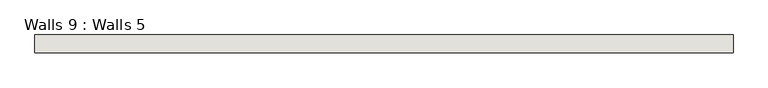
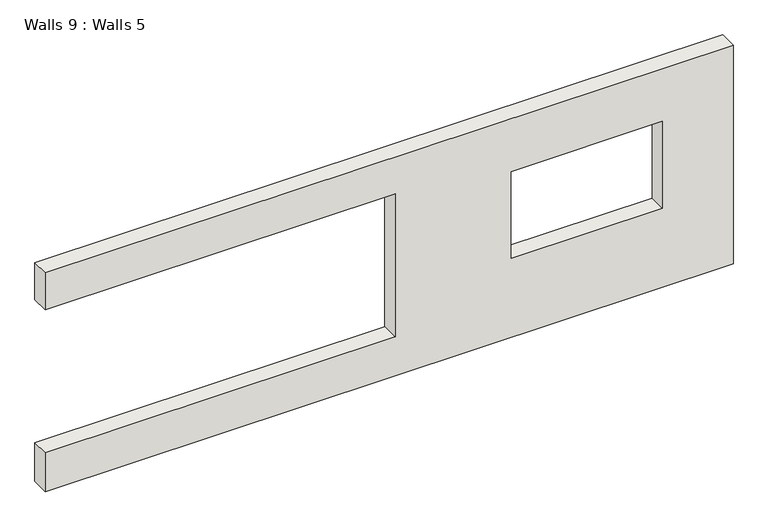
"""IFC4 building model written with IfcOpenShell, lengths in millimetres: wall geometry, Walls 9 : Walls 5."""

from ifc_helpers import new_model, si_unit, frame, origin, place, context, project, spatial, polyline, outline, extrude, source, transform, mapped, element, save


def walls_9_walls_5_51837564(model_context):
    return source(origin(), model_context, "Body", "SweptSolid", [
        extrude(outline(polyline([(11277.6, 2924.6563456), (11277.6, -8860.5727738), (10610.6696768, -8860.5727738), (10610.6696768, -2866.5436544), (8019.8696768, -2866.5436544), (8019.8696768, -8860.5727738), (7315.2, -8860.5727738), (7315.2, 2924.6563456), (11277.6, 2924.6563456)]), holes=[polyline([(10319.3693979, 1712.6958607), (8744.5693979, 1712.6958607), (8744.5693979, -878.1041393), (10319.3693979, -878.1041393), (10319.3693979, 1712.6958607)])]), frame((0.0, -4294.0325754, 0.0), z_axis=(0.0, 1.0, 0.0), x_axis=(0.0, 0.0, 1.0)), (0.0, 0.0, 1.0), 304.8),
    ])


if __name__ == "__main__":
    model = new_model("IFC4")
    model_context = context("Model", 3, world=origin())
    ifc_project = project(units=[si_unit("LENGTHUNIT", "METRE", prefix="MILLI")], contexts=[model_context])
    site = spatial("IfcSite", under=ifc_project)
    building = spatial("IfcBuilding", under=site)
    placement = place(None, origin())
    walls_9_walls_5_shape = walls_9_walls_5_51837564(model_context)
    element("IfcWall", 1, ObjectType="Walls 9 : Walls 5", at=placement, inside=building, context=model_context, shape_type="MappedRepresentation", body=[
        mapped(walls_9_walls_5_shape, transform((0.0, 0.0, 0.0), x_axis=(1.0, 0.0, 0.0), y_axis=(0.0, 1.0, 0.0), z_axis=(0.0, 0.0, 1.0))),
    ])
    save(model, "model.ifc")

# Revit data of these elements
# Element 1 (IfcWall, "Walls 9 : Walls 5")
#   Materials on its faces: "Default Wall"
# Materials
#   "Default Wall": colour RGB 128 128 128, transparency 0
